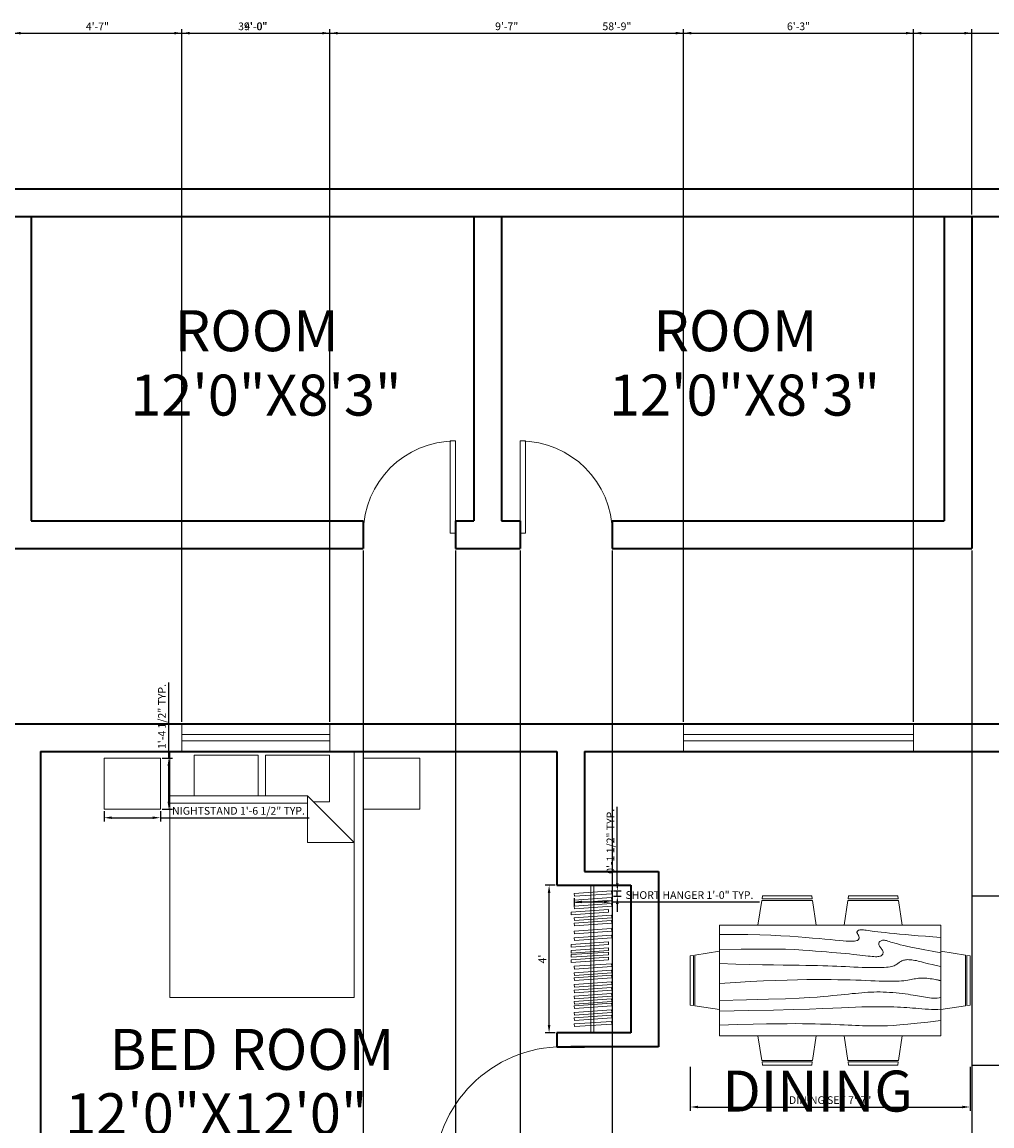
# Model space of a CAD drawing. Units: inches. Extents: x 3412 to 4225, y 13529 to 14581.
# Tile 5 of 7: x 3627 to 3943, y 14222 to 14581. Entities that reach past the tile are written whole.
import ezdxf

# ---------------------------------------------------------------- set-up
doc = ezdxf.new("R2010")
doc.units = ezdxf.units.IN
for name, color, linetype, lineweight in [('A-ANNO-DIMS', 2, 'Continuous', 13), ('A-AREA-IDEN', 7, 'Continuous', 18), ('A-DOOR', 4, 'Continuous', 18), ('A-FLOR-CASE', 9, 'Continuous', 18), ('A-FURN', 8, 'Continuous', 18), ('A-GLAZ', 4, 'Continuous', 13), ('A-WALL', 7, 'Continuous', 35), ('C-SITE-WALL', 7, 'Continuous', 35)]:
    doc.layers.add(name, color=color, linetype=linetype, lineweight=lineweight)
doc.styles.get("Standard").update_dxf_attribs({"font": 'arial.ttf'})
doc.dimstyles.new('ISO-25', dxfattribs={"dimtxt": 2.5, "dimasz": 2.5, "dimexe": 1.25, "dimexo": 0.625, "dimtad": 1, "dimdec": 0, "dimlunit": 3, "dimtxsty": 'Standard', "dimcen": 2.5, "dimadec": 0, "dimazin": 0, "dimtfac": 1, "dimtdec": 0, "dimtmove": 0, "dimatfit": 3, "dimfxl": 1, "dimarcsym": 0})

# ---------------------------------------------------------------- blocks, each defined once
blk = doc.blocks.new('*U3')
for p, q in [((0, 0), (0, -5)), ((30, 0), (30, -5))]:
    blk.add_line(p, q)
blk.add_lwpolyline([(0, 0), (0, 30), (1.75, 30), (1.75, 0)], close=True)
blk.add_arc((0, 0), 30, 0, 90)
blk = doc.blocks.new('Bed - Queen')
for p, q in [((0, -80.00003), (0, 0)), ((0, 0), (59.99999, 0)), ((59.99999, 0), (59.99999, -80.00003)), ((7.99999, -1.2), (28.79998, -1.2)), ((7.99999, -14.4), (7.99999, -1.2)), ((28.79998, -1.2), (28.79998, -14.4)), ((31.19999, -1.2), (51.99999, -1.2)), ((31.19999, -14.4), (31.19999, -1.2)), ((51.99999, -1.2), (51.99999, -16.4)), ((0, -14.4), (44.8, -14.4)), ((44.8, -16.8), (0, -16.8)), ((59.99999, -29.6), (44.8, -14.4)), ((44.8, -14.4), (44.8, -29.6)), ((51.99999, -16.4), (46.79936, -16.4)), ((44.8, -29.6), (59.99999, -29.6)), ((59.99999, -80.00003), (0, -80.00003))]:
    blk.add_line(p, q)
blk = doc.blocks.new('Dining Set - 36 x 72 in.')
for p, q in [((-22.2343, 26.00059), (-23.4847, 17.99762)), ((-22.2304, 26), (-5.7608, 26)), ((-22, 27.5), (-22.1562, 26.50042)), ((-5.8416, 26.5), (-22.1534, 26.5)), ((-22, 27.5), (-6, 27.5)), ((-5.8437, 26.49966), (-6, 27.5)), ((-4.5152, 17.99762), (-5.7655, 25.99926)), ((5.7657, 26.00059), (4.5153, 17.99762)), ((5.7696, 26), (22.2392, 26)), ((6, 27.5), (5.8438, 26.50042)), ((22.1584, 26.5), (5.8466, 26.5)), ((6, 27.5), (22, 27.5)), ((22.1563, 26.49966), (22, 27.5)), ((23.4848, 17.99762), (22.2345, 25.99926)), ((36, 18), (-36, 18)), ((-36, 18), (-36, -18)), ((36, -18), (36, 18)), ((-45.5, 8), (-44.5004, 8.15617)), ((-45.5, 8), (-45.5, -8)), ((-44.5, -8.15843), (-44.5, 8.15338)), ((-44.0006, 8.23428), (-35.9976, 9.48474)), ((-44, 8.23041), (-44, -8.23915)), ((44.0006, 8.23428), (35.9976, 9.48474)), ((44, 8.23041), (44, -8.23915)), ((44.5, -8.15843), (44.5, 8.15338)), ((45.5, 8), (44.5005, 8.15617)), ((45.5, 8), (45.5, -8)), ((-44.4997, -8.15631), (-45.5, -8)), ((-35.9976, -9.48476), (-43.9993, -8.2345)), ((35.9976, -9.48476), (43.9993, -8.2345)), ((44.4997, -8.15631), (45.5, -8)), ((-36, -18), (36, -18)), ((-22.2343, -26.0006), (-23.4847, -17.99762)), ((-4.5152, -17.99762), (-5.7655, -25.99928)), ((5.7657, -26.0006), (4.5153, -17.99762)), ((23.4848, -17.99762), (22.2345, -25.99928)), ((-22.2304, -26), (-5.7608, -26)), ((-22, -27.5), (-22.1562, -26.50044)), ((-5.8416, -26.5), (-22.1534, -26.5)), ((-22, -27.5), (-6, -27.5)), ((-5.8437, -26.49967), (-6, -27.5)), ((5.7696, -26), (22.2392, -26)), ((6, -27.5), (5.8438, -26.50044)), ((22.1584, -26.5), (5.8466, -26.5)), ((6, -27.5), (22, -27.5)), ((22.1563, -26.49967), (22, -27.5))]:
    blk.add_line(p, q)
for points in [[(-36, 15), (-31.1772, 14.97754), (-26.8079, 14.91406), (-22.8538, 14.81543), (-19.276, 14.6875), (-16.0362, 14.53613), (-13.0957, 14.36718), (-10.4159, 14.18652), (-7.9583, 14), (-5.6904, 13.81315), (-3.6035, 13.63021), (-1.6954, 13.45508), (0.0365, 13.29166), (1.5945, 13.14388), (2.9811, 13.01562), (4.1988, 12.9108), (5.25, 12.83333), (6.1393, 12.78613), (6.8802, 12.76823), (7.4883, 12.77767), (7.9792, 12.8125), (8.3685, 12.87077), (8.6719, 12.95052), (8.9049, 13.0498), (9.0833, 13.16666), (9.2205, 13.29899), (9.3216, 13.44401), (9.3895, 13.59879), (9.4271, 13.76041), (9.4373, 13.92594), (9.4232, 14.09245), (9.3875, 14.257), (9.3333, 14.41666), (9.2638, 14.56917), (9.1836, 14.71484), (9.0975, 14.85465), (9.0104, 14.98958), (8.9272, 15.1206), (8.8529, 15.2487), (8.7922, 15.37483), (8.75, 15.5), (8.7305, 15.62467), (8.7344, 15.74739), (8.7617, 15.86621), (8.8125, 15.97916), (8.8867, 16.08431), (8.9844, 16.17968), (9.1055, 16.26334), (9.25, 16.33333), (9.4189, 16.38802), (9.6172, 16.42708), (9.8506, 16.45052), (10.125, 16.45833), (10.4463, 16.45052), (10.8203, 16.42708), (11.2529, 16.38802), (11.75, 16.33333), (12.3184, 16.26318), (12.9694, 16.17838), (13.7151, 16.07991), (14.5677, 15.96875), (15.5395, 15.84586), (16.6426, 15.71224), (17.8893, 15.56884), (19.2917, 15.41666), (20.859, 15.25667), (22.5879, 15.08984), (24.4721, 14.91715), (26.5052, 14.73958), (28.6809, 14.5581), (30.9929, 14.3737), (33.4347, 14.18733), (36, 14)], [(-36, 10), (-28.9766, 10.14274), (-23.1725, 10.20442), (-18.4241, 10.19775), (-14.5677, 10.13541), (-11.4399, 10.03011), (-8.877, 9.89453), (-6.7154, 9.74137), (-4.7917, 9.58333), (-2.9698, 9.43082), (-1.2246, 9.28515), (0.4415, 9.14534), (2.026, 9.01041), (3.5266, 8.87939), (4.9408, 8.7513), (6.266, 8.62516), (7.5, 8.5), (8.6411, 8.37549), (9.6914, 8.2539), (10.6538, 8.13818), (11.5312, 8.03125), (12.3267, 7.93603), (13.043, 7.85547), (13.6831, 7.79248), (14.25, 7.75), (14.7471, 7.7303), (15.1797, 7.73307), (15.5537, 7.75732), (15.875, 7.80208), (16.1494, 7.86637), (16.3828, 7.94922), (16.5811, 8.04964), (16.75, 8.16666), (16.8944, 8.29915), (17.0143, 8.44531), (17.1089, 8.60319), (17.1771, 8.77083), (17.218, 8.94629), (17.2305, 9.1276), (17.2137, 9.31282), (17.1667, 9.5), (17.0895, 9.6875), (16.987, 9.875), (16.8649, 10.0625), (16.7292, 10.25), (16.5856, 10.4375), (16.4401, 10.625), (16.2985, 10.8125), (16.1667, 11), (16.05, 11.18733), (15.9518, 11.3737), (15.8752, 11.5581), (15.8229, 11.73958), (15.798, 11.91715), (15.8034, 12.08984), (15.842, 12.25667), (15.9167, 12.41666), (16.0295, 12.56836), (16.1784, 12.70833), (16.3605, 12.83268), (16.5729, 12.9375), (16.8127, 13.01888), (17.0768, 13.07291), (17.3625, 13.0957), (17.6667, 13.08333), (17.9894, 13.03312), (18.3418, 12.94726), (18.7382, 12.82918), (19.1927, 12.68229), (19.7195, 12.51001), (20.3327, 12.31575), (21.0465, 12.10294), (21.875, 11.875), (22.8357, 11.63354), (23.959, 11.37304), (25.2786, 11.08618), (26.8282, 10.76562), (28.6414, 10.40405), (30.752, 9.99414), (33.1936, 9.52856), (36, 9)], [(-36, 5.5), (-30.7157, 5.3348), (-26.069, 5.20963), (-21.9946, 5.11767), (-18.4271, 5.05208), (-15.3009, 5.00602), (-12.5508, 4.97265), (-10.1112, 4.94515), (-7.9167, 4.91666), (-5.909, 4.88167), (-4.0586, 4.83984), (-2.3429, 4.79215), (-0.7396, 4.73958), (0.7739, 4.6831), (2.22, 4.6237), (3.6213, 4.56233), (5, 4.5), (6.373, 4.43782), (7.7344, 4.3776), (9.0723, 4.32129), (10.375, 4.27083), (11.6309, 4.22819), (12.8281, 4.19531), (13.9551, 4.17415), (15, 4.16666), (15.954, 4.17448), (16.819, 4.19791), (17.6001, 4.23698), (18.3021, 4.29166), (18.9299, 4.36198), (19.4883, 4.44791), (19.9823, 4.54948), (20.4167, 4.66666), (20.7969, 4.79899), (21.1302, 4.94401), (21.4245, 5.09879), (21.6875, 5.26041), (21.9271, 5.42594), (22.1511, 5.59245), (22.3672, 5.757), (22.5834, 5.91666), (22.8065, 6.06868), (23.0404, 6.21093), (23.2879, 6.34147), (23.5521, 6.45833), (23.8358, 6.55957), (24.142, 6.64323), (24.4735, 6.70735), (24.8334, 6.75), (25.2235, 6.76969), (25.642, 6.76692), (26.0858, 6.74267), (26.5521, 6.69791), (27.0379, 6.63362), (27.5404, 6.55078), (28.0565, 6.45036), (28.5834, 6.33333), (29.1242, 6.19987), (29.7071, 6.04687), (30.3661, 5.87044), (31.1354, 5.66666), (32.0493, 5.43164), (33.142, 5.16146), (34.4475, 4.85221), (36, 4.5)], [(-36, -1), (-30.7915, -0.6591), (-26.0195, -0.38216), (-21.6519, -0.16284), (-17.6563, 0.00521), (-14.0005, 0.12833), (-10.6523, 0.21289), (-7.5796, 0.26522), (-4.75, 0.29166), (-2.134, 0.29793), (0.2878, 0.28711), (2.5317, 0.26163), (4.6146, 0.22396), (6.5529, 0.17651), (8.3633, 0.12174), (10.0623, 0.06209), (11.6667, 0), (13.1899, -0.06201), (14.6341, -0.1211), (15.9982, -0.17432), (17.2813, -0.21875), (18.4823, -0.25147), (19.6003, -0.26953), (20.6343, -0.27002), (21.5834, -0.25), (22.4481, -0.20768), (23.2357, -0.14584), (23.9549, -0.06836), (24.6146, 0.02083), (25.2235, 0.11784), (25.7904, 0.21875), (26.3241, 0.31966), (26.8334, 0.41666), (27.3265, 0.50618), (27.8099, 0.58593), (28.2894, 0.65397), (28.7709, 0.70833), (29.2601, 0.74707), (29.763, 0.76823), (30.2855, 0.76985), (30.8334, 0.75), (31.4088, 0.70784), (31.9994, 0.64713), (32.589, 0.57275), (33.1615, 0.48958), (33.7008, 0.4025), (34.1908, 0.3164), (34.6153, 0.23616), (34.9584, 0.16666), (35.2099, 0.11165), (35.3848, 0.07031), (35.504, 0.04069), (35.5886, 0.02083), (35.6594, 0.00879), (35.7377, 0.0026), (35.8442, 0.00032), (36, 0)], [(-36, -6.5), (-27.1843, -6.31267), (-20.084, -6.1263), (-14.469, -5.9419), (-10.1094, -5.76042), (-6.7752, -5.58285), (-4.2363, -5.41016), (-2.2629, -5.24333), (-0.625, -5.08334), (0.8708, -4.93099), (2.2715, -4.78646), (3.5872, -4.64974), (4.8281, -4.52084), (6.0046, -4.39974), (7.127, -4.28646), (8.2053, -4.18099), (9.25, -4.08334), (10.2705, -3.99382), (11.2734, -3.91407), (12.2647, -3.84603), (13.25, -3.79167), (14.2354, -3.75293), (15.2266, -3.73177), (16.2295, -3.73015), (17.25, -3.75), (18.2912, -3.79248), (19.3451, -3.85547), (20.4009, -3.93604), (21.4479, -4.03125), (22.4754, -4.13819), (23.4727, -4.25391), (24.4289, -4.37549), (25.3334, -4.5), (26.1785, -4.62492), (26.9694, -4.74935), (27.7145, -4.87281), (28.4219, -4.99479), (29.1, -5.11483), (29.7572, -5.23242), (30.4016, -5.34709), (31.0417, -5.45834), (31.6837, -5.56437), (32.3262, -5.65821), (32.9658, -5.73153), (33.599, -5.77604), (34.2224, -5.78345), (34.8327, -5.74545), (35.4264, -5.65373), (36, -5.5)], [(-36, -10), (-26.4022, -9.81299), (-18.4675, -9.62891), (-11.9839, -9.45069), (-6.7396, -9.28125), (-2.5226, -9.12354), (0.8789, -8.98047), (3.6769, -8.85498), (6.0833, -8.75), (8.2767, -8.66765), (10.3021, -8.60677), (12.1712, -8.56543), (13.8958, -8.54167), (15.4876, -8.53353), (16.9583, -8.53907), (18.3197, -8.55632), (19.5834, -8.58334), (20.7616, -8.61841), (21.8685, -8.66081), (22.9188, -8.71004), (23.9271, -8.76563), (24.9081, -8.82707), (25.8763, -8.89388), (26.8465, -8.96558), (27.8334, -9.04167), (28.8474, -9.12118), (29.8828, -9.20117), (30.93, -9.27824), (31.9792, -9.34896), (33.0205, -9.40991), (34.0443, -9.45768), (35.0407, -9.48885), (36, -9.5)], [(-36, -14.5), (-30.0881, -14.33513), (-25.0332, -14.21224), (-20.7312, -14.12647), (-17.0781, -14.07292), (-13.97, -14.04671), (-11.3027, -14.04297), (-8.9724, -14.05681), (-6.875, -14.08334), (-4.9224, -14.11833), (-3.0905, -14.16016), (-1.3709, -14.20785), (0.2448, -14.26042), (1.7647, -14.3169), (3.1973, -14.3763), (4.5507, -14.43767), (5.8333, -14.5), (7.0554, -14.5621), (8.235, -14.62175), (9.3922, -14.67652), (10.5469, -14.72396), (11.7192, -14.76164), (12.929, -14.78711), (14.1965, -14.79794), (15.5417, -14.79167), (16.9933, -14.76424), (18.6152, -14.70508), (20.4804, -14.60197), (22.6615, -14.44271), (25.2312, -14.21509), (28.2624, -13.9069), (31.8277, -13.50594), (36, -13)]]:
    blk.add_lwpolyline(points)
blk = doc.blocks.new('*D15')
at = {"layer": 'A-ANNO-DIMS', "color": 0, "lineweight": -2, "transparency": 16777216}
for p, q in [((3800.73, 14299.93), (3797.55, 14299.93)), ((3798.8, 14254.43), (3798.8, 14297.43)), ((3800.73, 14251.93), (3797.55, 14251.93))]:
    blk.add_line(p, q, dxfattribs=at)
at = {"layer": 'A-ANNO-DIMS', "color": 0, "transparency": 16777216}
for points in [[(3798.38, 14297.43), (3799.21, 14297.43), (3798.8, 14299.93)], [(3798.38, 14254.43), (3799.21, 14254.43), (3798.8, 14251.93)]]:
    blk.add_solid(points, dxfattribs=at)
at = {"layer": 'Defpoints', "color": 0, "transparency": 16777216}
for p in [(3798.8, 14299.93), (3801.36, 14299.93), (3801.36, 14251.93)]:
    blk.add_point(p, dxfattribs=at)
at = {"layer": 'A-ANNO-DIMS', "color": 0, "transparency": 16777216, "insert": (3796.92, 14275.93), "char_height": 2.5, "attachment_point": 5, "rotation": 90}
blk.add_mtext("4'", dxfattribs=at)
blk = doc.blocks.new('NIGHTSTAND')
blk.add_lwpolyline([(0, 16.62), (18.31, 16.62), (18.31, 0), (0, 0)], close=True)
blk = doc.blocks.new('CLOSET-HANGER-SHORT')
blk.add_lwpolyline([(0, 0.87), (12.13, 1.73), (12.19, 0.86), (0.06, 0)], close=True)
blk = doc.blocks.new('*D36')
at = {"layer": 'A-ANNO-DIMS', "color": 0, "lineweight": -2, "transparency": 16777216}
for p, q in [((3654.03, 14324.02), (3654.03, 14320.64)), ((3672.34, 14324.02), (3672.34, 14320.64)), ((3656.53, 14321.89), (3669.84, 14321.89)), ((3672.34, 14321.89), (3720.71, 14321.89))]:
    blk.add_line(p, q, dxfattribs=at)
at = {"layer": 'A-ANNO-DIMS', "color": 0, "transparency": 16777216}
for points in [[(3656.53, 14322.31), (3656.53, 14321.48), (3654.03, 14321.89)], [(3669.84, 14322.31), (3669.84, 14321.48), (3672.34, 14321.89)]]:
    blk.add_solid(points, dxfattribs=at)
at = {"layer": 'Defpoints', "color": 0, "transparency": 16777216}
for p in [(3654.03, 14324.64), (3672.34, 14324.64), (3672.34, 14321.89)]:
    blk.add_point(p, dxfattribs=at)
at = {"layer": 'A-ANNO-DIMS', "color": 0, "transparency": 16777216, "insert": (3697.77, 14323.81), "char_height": 2.5, "attachment_point": 5}
blk.add_mtext('NIGHTSTAND 1\'-6 1/2" TYP.', dxfattribs=at)
blk = doc.blocks.new('*D37')
at = {"layer": 'A-ANNO-DIMS', "color": 0, "lineweight": -2, "transparency": 16777216}
for p, q in [((3675.09, 14341.26), (3675.09, 14365.84)), ((3672.97, 14341.26), (3676.34, 14341.26)), ((3675.09, 14327.14), (3675.09, 14338.76)), ((3672.97, 14324.64), (3676.34, 14324.64))]:
    blk.add_line(p, q, dxfattribs=at)
at = {"layer": 'A-ANNO-DIMS', "color": 0, "transparency": 16777216}
for points in [[(3674.67, 14338.76), (3675.5, 14338.76), (3675.09, 14341.26)], [(3674.67, 14327.14), (3675.5, 14327.14), (3675.09, 14324.64)]]:
    blk.add_solid(points, dxfattribs=at)
at = {"layer": 'Defpoints', "color": 0, "transparency": 16777216}
for p in [(3672.34, 14341.26), (3675.09, 14341.26), (3672.34, 14324.64)]:
    blk.add_point(p, dxfattribs=at)
at = {"layer": 'A-ANNO-DIMS', "color": 0, "transparency": 16777216, "insert": (3673.17, 14354.8), "char_height": 2.5, "attachment_point": 5, "rotation": 90}
blk.add_mtext('1\'-4 1/2" TYP.', dxfattribs=at)
blk = doc.blocks.new('*D42')
at = {"layer": 'A-ANNO-DIMS', "color": 0, "lineweight": -2, "transparency": 16777216}
for p, q in [((3806.97, 14295.71), (3806.97, 14293.26)), ((3809.47, 14294.51), (3816.66, 14294.51)), ((3819.16, 14295.71), (3819.16, 14293.26)), ((3819.16, 14294.51), (3867.25, 14294.51))]:
    blk.add_line(p, q, dxfattribs=at)
at = {"layer": 'A-ANNO-DIMS', "color": 0, "transparency": 16777216}
for points in [[(3809.47, 14294.92), (3809.47, 14294.09), (3806.97, 14294.51)], [(3816.66, 14294.92), (3816.66, 14294.09), (3819.16, 14294.51)]]:
    blk.add_solid(points, dxfattribs=at)
at = {"layer": 'Defpoints', "color": 0, "transparency": 16777216}
for p in [(3806.97, 14296.33), (3819.16, 14296.33), (3819.16, 14294.51)]:
    blk.add_point(p, dxfattribs=at)
at = {"layer": 'A-ANNO-DIMS', "color": 0, "transparency": 16777216, "insert": (3844.45, 14296.42), "char_height": 2.5, "attachment_point": 5}
blk.add_mtext('SHORT HANGER 1\'-0" TYP.', dxfattribs=at)
blk = doc.blocks.new('*D43')
at = {"layer": 'A-ANNO-DIMS', "color": 0, "lineweight": -2, "transparency": 16777216}
for p, q in [((3820.99, 14300.57), (3820.99, 14325.38)), ((3819.79, 14298.07), (3822.24, 14298.07)), ((3819.79, 14296.33), (3822.24, 14296.33)), ((3820.99, 14296.33), (3820.99, 14298.07)), ((3820.99, 14293.83), (3820.99, 14291.33))]:
    blk.add_line(p, q, dxfattribs=at)
at = {"layer": 'A-ANNO-DIMS', "color": 0, "transparency": 16777216}
for points in [[(3820.57, 14300.57), (3821.41, 14300.57), (3820.99, 14298.07)], [(3820.57, 14293.83), (3821.41, 14293.83), (3820.99, 14296.33)]]:
    blk.add_solid(points, dxfattribs=at)
at = {"layer": 'Defpoints', "color": 0, "transparency": 16777216}
for p in [(3819.16, 14298.07), (3819.16, 14296.33), (3820.99, 14298.07)]:
    blk.add_point(p, dxfattribs=at)
at = {"layer": 'A-ANNO-DIMS', "color": 0, "transparency": 16777216, "insert": (3819.07, 14314.22), "char_height": 2.5, "attachment_point": 5, "rotation": 90}
blk.add_mtext('0\'-1 1/2" TYP.', dxfattribs=at)
blk = doc.blocks.new('*D52')
at = {"layer": 'A-ANNO-DIMS', "color": 0, "lineweight": -2, "transparency": 16777216}
for p, q in [((3844.72, 14240.84), (3844.72, 14226.56)), ((3935.72, 14240.84), (3935.72, 14226.56)), ((3847.22, 14227.81), (3933.22, 14227.81))]:
    blk.add_line(p, q, dxfattribs=at)
at = {"layer": 'A-ANNO-DIMS', "color": 0, "transparency": 16777216}
for points in [[(3847.22, 14228.23), (3847.22, 14227.4), (3844.72, 14227.81)], [(3933.22, 14228.23), (3933.22, 14227.4), (3935.72, 14227.81)]]:
    blk.add_solid(points, dxfattribs=at)
at = {"layer": 'Defpoints', "color": 0, "transparency": 16777216}
for p in [(3844.72, 14241.46), (3935.72, 14241.46), (3935.72, 14227.81)]:
    blk.add_point(p, dxfattribs=at)
at = {"layer": 'A-ANNO-DIMS', "color": 0, "transparency": 16777216, "insert": (3890.22, 14229.73), "char_height": 2.5, "attachment_point": 5}
blk.add_mtext('DINING SET 7\'-7"', dxfattribs=at)
blk = doc.blocks.new('*D53')
at = {"layer": 'A-ANNO-DIMS', "color": 0, "lineweight": -2, "transparency": 16777216}
for p, q in [((3936.34, 14296.46), (3950.62, 14296.46)), ((3949.37, 14243.96), (3949.37, 14293.96)), ((3936.34, 14241.46), (3950.62, 14241.46))]:
    blk.add_line(p, q, dxfattribs=at)
at = {"layer": 'A-ANNO-DIMS', "color": 0, "transparency": 16777216}
for points in [[(3948.95, 14293.96), (3949.79, 14293.96), (3949.37, 14296.46)], [(3948.95, 14243.96), (3949.79, 14243.96), (3949.37, 14241.46)]]:
    blk.add_solid(points, dxfattribs=at)
at = {"layer": 'Defpoints', "color": 0, "transparency": 16777216}
for p in [(3935.72, 14296.46), (3949.37, 14296.46), (3935.72, 14241.46)]:
    blk.add_point(p, dxfattribs=at)
at = {"layer": 'A-ANNO-DIMS', "color": 0, "transparency": 16777216, "insert": (3947.49, 14268.96), "char_height": 2.5, "attachment_point": 5, "rotation": 90}
blk.add_mtext('4\'-7"', dxfattribs=at)
blk = doc.blocks.new('*D56')
at = {"layer": 'A-ANNO-DIMS', "color": 0, "lineweight": -2, "transparency": 16777216}
for p, q in [((3468.36, 14527.06), (3468.36, 14578.28)), ((4173.36, 14527.06), (4173.36, 14578.28)), ((3470.86, 14577.03), (4170.86, 14577.03))]:
    blk.add_line(p, q, dxfattribs=at)
at = {"layer": 'A-ANNO-DIMS', "color": 0, "transparency": 16777216}
for points in [[(3470.86, 14577.45), (3470.86, 14576.62), (3468.36, 14577.03)], [(4170.86, 14577.45), (4170.86, 14576.62), (4173.36, 14577.03)]]:
    blk.add_solid(points, dxfattribs=at)
at = {"layer": 'Defpoints', "color": 0, "transparency": 16777216}
for p in [(4173.36, 14577.03), (3468.36, 14526.43), (4173.36, 14526.43)]:
    blk.add_point(p, dxfattribs=at)
at = {"layer": 'A-ANNO-DIMS', "color": 0, "transparency": 16777216, "insert": (3820.86, 14578.93), "char_height": 2.5, "attachment_point": 5}
blk.add_mtext('58\'-9"', dxfattribs=at)
blk = doc.blocks.new('*D59')
at = {"layer": 'A-ANNO-DIMS', "color": 0, "lineweight": -2, "transparency": 16777216}
for p, q in [((3468.36, 14527.06), (3468.36, 14578.28)), ((3936.36, 14518.06), (3936.36, 14578.28)), ((3470.86, 14577.03), (3933.86, 14577.03))]:
    blk.add_line(p, q, dxfattribs=at)
at = {"layer": 'A-ANNO-DIMS', "color": 0, "transparency": 16777216}
for points in [[(3470.86, 14577.45), (3470.86, 14576.62), (3468.36, 14577.03)], [(3933.86, 14577.45), (3933.86, 14576.62), (3936.36, 14577.03)]]:
    blk.add_solid(points, dxfattribs=at)
at = {"layer": 'Defpoints', "color": 0, "transparency": 16777216}
for p in [(3936.36, 14577.03), (3468.36, 14526.43), (3936.36, 14517.43)]:
    blk.add_point(p, dxfattribs=at)
at = {"layer": 'A-ANNO-DIMS', "color": 0, "transparency": 16777216, "insert": (3702.36, 14578.93), "char_height": 2.5, "attachment_point": 5}
blk.add_mtext('39\'-0"', dxfattribs=at)
blk = doc.blocks.new('*D63')
at = {"layer": 'A-ANNO-DIMS', "color": 0, "lineweight": -2, "transparency": 16777216}
for p, q in [((3615.36, 14408.81), (3615.36, 13550.58)), ((3738.36, 14408.81), (3738.36, 13550.58)), ((3617.86, 13551.83), (3735.86, 13551.83))]:
    blk.add_line(p, q, dxfattribs=at)
at = {"layer": 'A-ANNO-DIMS', "color": 0, "transparency": 16777216}
for points in [[(3617.86, 13552.25), (3617.86, 13551.42), (3615.36, 13551.83)], [(3735.86, 13552.25), (3735.86, 13551.42), (3738.36, 13551.83)]]:
    blk.add_solid(points, dxfattribs=at)
at = {"layer": 'Defpoints', "color": 0, "transparency": 16777216}
for p in [(3615.36, 14409.43), (3738.36, 14409.43), (3738.36, 13551.83)]:
    blk.add_point(p, dxfattribs=at)
at = {"layer": 'A-ANNO-DIMS', "color": 0, "transparency": 16777216, "insert": (3676.86, 13553.73), "char_height": 2.5, "attachment_point": 5}
blk.add_mtext('10\'-3"', dxfattribs=at)
blk = doc.blocks.new('*D64')
at = {"layer": 'A-ANNO-DIMS', "color": 0, "lineweight": -2, "transparency": 16777216}
for p, q in [((3738.36, 14408.81), (3738.36, 13550.58)), ((3768.36, 14408.81), (3768.36, 13550.58)), ((3740.86, 13551.83), (3765.86, 13551.83))]:
    blk.add_line(p, q, dxfattribs=at)
at = {"layer": 'A-ANNO-DIMS', "color": 0, "transparency": 16777216}
for points in [[(3740.86, 13552.25), (3740.86, 13551.42), (3738.36, 13551.83)], [(3765.86, 13552.25), (3765.86, 13551.42), (3768.36, 13551.83)]]:
    blk.add_solid(points, dxfattribs=at)
at = {"layer": 'Defpoints', "color": 0, "transparency": 16777216}
for p in [(3738.36, 14409.43), (3768.36, 14409.43), (3768.36, 13551.83)]:
    blk.add_point(p, dxfattribs=at)
at = {"layer": 'A-ANNO-DIMS', "color": 0, "transparency": 16777216, "insert": (3753.36, 13553.73), "char_height": 2.5, "attachment_point": 5}
blk.add_mtext('2\'-6"', dxfattribs=at)
blk = doc.blocks.new('*D65')
at = {"layer": 'A-ANNO-DIMS', "color": 0, "lineweight": -2, "transparency": 16777216}
for p, q in [((3768.36, 14408.81), (3768.36, 13550.58)), ((3789.36, 14408.81), (3789.36, 13550.58)), ((3770.86, 13551.83), (3786.86, 13551.83))]:
    blk.add_line(p, q, dxfattribs=at)
at = {"layer": 'A-ANNO-DIMS', "color": 0, "transparency": 16777216}
for points in [[(3770.86, 13552.25), (3770.86, 13551.42), (3768.36, 13551.83)], [(3786.86, 13552.25), (3786.86, 13551.42), (3789.36, 13551.83)]]:
    blk.add_solid(points, dxfattribs=at)
at = {"layer": 'Defpoints', "color": 0, "transparency": 16777216}
for p in [(3768.36, 14409.43), (3789.36, 14409.43), (3789.36, 13551.83)]:
    blk.add_point(p, dxfattribs=at)
at = {"layer": 'A-ANNO-DIMS', "color": 0, "transparency": 16777216, "insert": (3778.86, 13553.73), "char_height": 2.5, "attachment_point": 5}
blk.add_mtext('1\'-9"', dxfattribs=at)
blk = doc.blocks.new('*D66')
at = {"layer": 'A-ANNO-DIMS', "color": 0, "lineweight": -2, "transparency": 16777216}
for p, q in [((3789.36, 14408.81), (3789.36, 13550.58)), ((3819.36, 14408.81), (3819.36, 13550.58)), ((3791.86, 13551.83), (3816.86, 13551.83))]:
    blk.add_line(p, q, dxfattribs=at)
at = {"layer": 'A-ANNO-DIMS', "color": 0, "transparency": 16777216}
for points in [[(3791.86, 13552.25), (3791.86, 13551.42), (3789.36, 13551.83)], [(3816.86, 13552.25), (3816.86, 13551.42), (3819.36, 13551.83)]]:
    blk.add_solid(points, dxfattribs=at)
at = {"layer": 'Defpoints', "color": 0, "transparency": 16777216}
for p in [(3789.36, 14409.43), (3819.36, 14409.43), (3819.36, 13551.83)]:
    blk.add_point(p, dxfattribs=at)
at = {"layer": 'A-ANNO-DIMS', "color": 0, "transparency": 16777216, "insert": (3804.36, 13553.73), "char_height": 2.5, "attachment_point": 5}
blk.add_mtext('2\'-6"', dxfattribs=at)
blk = doc.blocks.new('*D67')
at = {"layer": 'A-ANNO-DIMS', "color": 0, "lineweight": -2, "transparency": 16777216}
for p, q in [((3819.36, 14408.81), (3819.36, 13550.58)), ((3936.36, 14408.81), (3936.36, 13550.58)), ((3821.86, 13551.83), (3933.86, 13551.83))]:
    blk.add_line(p, q, dxfattribs=at)
at = {"layer": 'A-ANNO-DIMS', "color": 0, "transparency": 16777216}
for points in [[(3821.86, 13552.25), (3821.86, 13551.42), (3819.36, 13551.83)], [(3933.86, 13552.25), (3933.86, 13551.42), (3936.36, 13551.83)]]:
    blk.add_solid(points, dxfattribs=at)
at = {"layer": 'Defpoints', "color": 0, "transparency": 16777216}
for p in [(3819.36, 14409.43), (3936.36, 14409.43), (3936.36, 13551.83)]:
    blk.add_point(p, dxfattribs=at)
at = {"layer": 'A-ANNO-DIMS', "color": 0, "transparency": 16777216, "insert": (3877.86, 13553.73), "char_height": 2.5, "attachment_point": 5}
blk.add_mtext('9\'-9"', dxfattribs=at)
blk = doc.blocks.new('*D68')
at = {"layer": 'A-ANNO-DIMS', "color": 0, "lineweight": -2, "transparency": 16777216}
for p, q in [((3624.36, 14353.06), (3624.36, 14578.28)), ((3679.38, 14353.06), (3679.38, 14578.28)), ((3626.86, 14577.03), (3676.88, 14577.03))]:
    blk.add_line(p, q, dxfattribs=at)
at = {"layer": 'A-ANNO-DIMS', "color": 0, "transparency": 16777216}
for points in [[(3626.86, 14577.45), (3626.86, 14576.62), (3624.36, 14577.03)], [(3676.88, 14577.45), (3676.88, 14576.62), (3679.38, 14577.03)]]:
    blk.add_solid(points, dxfattribs=at)
at = {"layer": 'Defpoints', "color": 0, "transparency": 16777216}
for p in [(3679.38, 14577.03), (3624.36, 14352.43), (3679.38, 14352.43)]:
    blk.add_point(p, dxfattribs=at)
at = {"layer": 'A-ANNO-DIMS', "color": 0, "transparency": 16777216, "insert": (3651.87, 14578.91), "char_height": 2.5, "attachment_point": 5}
blk.add_mtext('4\'-7"', dxfattribs=at)
blk = doc.blocks.new('*D69')
at = {"layer": 'A-ANNO-DIMS', "color": 0, "lineweight": -2, "transparency": 16777216}
for p, q in [((3679.38, 14353.06), (3679.38, 14578.28)), ((3727.48, 14353.06), (3727.48, 14578.28)), ((3681.88, 14577.03), (3724.98, 14577.03))]:
    blk.add_line(p, q, dxfattribs=at)
at = {"layer": 'A-ANNO-DIMS', "color": 0, "transparency": 16777216}
for points in [[(3681.88, 14577.45), (3681.88, 14576.62), (3679.38, 14577.03)], [(3724.98, 14577.45), (3724.98, 14576.62), (3727.48, 14577.03)]]:
    blk.add_solid(points, dxfattribs=at)
at = {"layer": 'Defpoints', "color": 0, "transparency": 16777216}
for p in [(3727.48, 14577.03), (3679.38, 14352.43), (3727.48, 14352.43)]:
    blk.add_point(p, dxfattribs=at)
at = {"layer": 'A-ANNO-DIMS', "color": 0, "transparency": 16777216, "insert": (3703.43, 14578.93), "char_height": 2.5, "attachment_point": 5}
blk.add_mtext('4\'-0"', dxfattribs=at)
blk = doc.blocks.new('*D70')
at = {"layer": 'A-ANNO-DIMS', "color": 0, "lineweight": -2, "transparency": 16777216}
for p, q in [((3727.48, 14353.06), (3727.48, 14578.28)), ((3842.52, 14353.06), (3842.52, 14578.28)), ((3729.98, 14577.03), (3840.02, 14577.03))]:
    blk.add_line(p, q, dxfattribs=at)
at = {"layer": 'A-ANNO-DIMS', "color": 0, "transparency": 16777216}
for points in [[(3729.98, 14577.45), (3729.98, 14576.62), (3727.48, 14577.03)], [(3840.02, 14577.45), (3840.02, 14576.62), (3842.52, 14577.03)]]:
    blk.add_solid(points, dxfattribs=at)
at = {"layer": 'Defpoints', "color": 0, "transparency": 16777216}
for p in [(3842.52, 14577.03), (3727.48, 14352.43), (3842.52, 14352.43)]:
    blk.add_point(p, dxfattribs=at)
at = {"layer": 'A-ANNO-DIMS', "color": 0, "transparency": 16777216, "insert": (3785, 14578.93), "char_height": 2.5, "attachment_point": 5}
blk.add_mtext('9\'-7"', dxfattribs=at)
blk = doc.blocks.new('*D71')
at = {"layer": 'A-ANNO-DIMS', "color": 0, "lineweight": -2, "transparency": 16777216}
for p, q in [((3842.52, 14353.06), (3842.52, 14578.28)), ((3917.36, 14353.06), (3917.36, 14578.28)), ((3845.02, 14577.03), (3914.86, 14577.03))]:
    blk.add_line(p, q, dxfattribs=at)
at = {"layer": 'A-ANNO-DIMS', "color": 0, "transparency": 16777216}
for points in [[(3845.02, 14577.45), (3845.02, 14576.62), (3842.52, 14577.03)], [(3914.86, 14577.45), (3914.86, 14576.62), (3917.36, 14577.03)]]:
    blk.add_solid(points, dxfattribs=at)
at = {"layer": 'Defpoints', "color": 0, "transparency": 16777216}
for p in [(3917.36, 14577.03), (3842.52, 14352.43), (3917.36, 14352.43)]:
    blk.add_point(p, dxfattribs=at)
at = {"layer": 'A-ANNO-DIMS', "color": 0, "transparency": 16777216, "insert": (3879.94, 14578.93), "char_height": 2.5, "attachment_point": 5}
blk.add_mtext('6\'-3"', dxfattribs=at)
blk = doc.blocks.new('*D72')
at = {"layer": 'A-ANNO-DIMS', "color": 0, "lineweight": -2, "transparency": 16777216}
for p, q in [((3917.36, 14353.06), (3917.36, 14578.28)), ((4092.36, 14353.06), (4092.36, 14578.28)), ((3919.86, 14577.03), (4089.86, 14577.03))]:
    blk.add_line(p, q, dxfattribs=at)
at = {"layer": 'A-ANNO-DIMS', "color": 0, "transparency": 16777216}
for points in [[(3919.86, 14577.45), (3919.86, 14576.62), (3917.36, 14577.03)], [(4089.86, 14577.45), (4089.86, 14576.62), (4092.36, 14577.03)]]:
    blk.add_solid(points, dxfattribs=at)
at = {"layer": 'Defpoints', "color": 0, "transparency": 16777216}
for p in [(4092.36, 14577.03), (3917.36, 14352.43), (4092.36, 14352.43)]:
    blk.add_point(p, dxfattribs=at)
at = {"layer": 'A-ANNO-DIMS', "color": 0, "transparency": 16777216, "insert": (4004.86, 14578.91), "char_height": 2.5, "attachment_point": 5}
blk.add_mtext('14\'-7"', dxfattribs=at)

msp = doc.modelspace()

# ---------------------------------------------------------------- linework, layer by layer
at = {"layer": 'A-FLOR-CASE'}
for p, q in [((3812.36, 14299.93), (3812.36, 14251.93)), ((3813.36, 14299.93), (3813.36, 14251.93))]:
    msp.add_line(p, q, dxfattribs=at)
at = {"layer": 'A-GLAZ'}
for p, q in [((3679.38, 14343.43), (3679.38, 14352.43)), ((3727.48, 14343.43), (3727.48, 14352.43)), ((3842.52, 14343.43), (3842.52, 14352.43)), ((3917.36, 14343.43), (3917.36, 14352.43)), ((3679.38, 14348.93), (3727.48, 14348.93)), ((3842.52, 14348.93), (3917.36, 14348.93)), ((3679.38, 14346.93), (3727.48, 14346.93)), ((3842.52, 14346.93), (3917.36, 14346.93))]:
    msp.add_line(p, q, dxfattribs=at)
at = {"layer": 'A-WALL'}
for p, q in [((3630.36, 14517.43), (3630.36, 14418.43)), ((3774.36, 14517.43), (3774.36, 14418.43)), ((3783.36, 14517.43), (3783.36, 14418.43)), ((3927.36, 14517.43), (3927.36, 14418.43)), ((3936.36, 14517.43), (3936.36, 14409.43)), ((3630.36, 14418.43), (3738.36, 14418.43)), ((3738.36, 14418.43), (3738.36, 14409.43)), ((3768.36, 14418.43), (3768.36, 14409.43)), ((3768.36, 14418.43), (3774.36, 14418.43)), ((3783.36, 14418.43), (3789.36, 14418.43)), ((3789.36, 14418.43), (3789.36, 14409.43)), ((3819.36, 14418.43), (3819.36, 14409.43)), ((3819.36, 14418.43), (3927.36, 14418.43)), ((3615.36, 14409.43), (3738.36, 14409.43)), ((3768.36, 14409.43), (3789.36, 14409.43)), ((3819.36, 14409.43), (3936.36, 14409.43)), ((3624.36, 14352.43), (4092.36, 14352.43)), ((3633.36, 14343.43), (3633.36, 14199.43)), ((3633.36, 14343.43), (3801.36, 14343.43)), ((3801.36, 14343.43), (3801.36, 14299.93)), ((3810.36, 14343.43), (3810.36, 14304.43)), ((3810.36, 14343.43), (3948.36, 14343.43)), ((3810.36, 14304.43), (3834.36, 14304.43)), ((3834.36, 14304.43), (3834.36, 14247.43)), ((3801.36, 14299.93), (3825.36, 14299.93)), ((3825.36, 14299.93), (3825.36, 14251.93)), ((3825.36, 14251.93), (3801.36, 14251.93)), ((3801.36, 14251.93), (3801.36, 14247.43)), ((3801.36, 14247.43), (3810.36, 14247.43)), ((3834.36, 14247.43), (3805.86, 14247.43))]:
    msp.add_line(p, q, dxfattribs=at)
at = {"layer": 'C-SITE-WALL'}
for p, q in [((3468.36, 14526.43), (4173.36, 14526.43)), ((3477.36, 14517.43), (4164.36, 14517.43))]:
    msp.add_line(p, q, dxfattribs=at)

# ---------------------------------------------------------------- block references
at = {"layer": 'A-DOOR', "xscale": -1}
msp.add_blockref('*U3', (3768.36, 14414.43), dxfattribs=at)
at = {"layer": 'A-DOOR'}
msp.add_blockref('*U3', (3789.36, 14414.43), dxfattribs=at)
at = {"layer": 'A-DOOR', "xscale": 1.399999999999999, "yscale": 1.399999999999999, "zscale": 1.399999999999999, "rotation": 89.99999999999999}
msp.add_blockref('*U3', (3803.36, 14205.43), dxfattribs=at)
at = {"layer": 'A-FLOR-CASE'}
for p in [(3806.97, 14296.33), (3806.97, 14294.21), (3805.97, 14290.33), (3806.97, 14292.29), (3806.97, 14288.49), (3806.97, 14286.72), (3806.97, 14284.17), (3805.97, 14279.75), (3806.97, 14281.93), (3805.97, 14277.89), (3805.97, 14276.49), (3805.97, 14274.8), (3806.97, 14272.69), (3806.97, 14270.63), (3806.97, 14268.94), (3806.97, 14266.79), (3806.97, 14264.97), (3806.97, 14263.04), (3806.97, 14261.25), (3806.97, 14259.83), (3806.97, 14257.73), (3806.97, 14255.99), (3806.97, 14253.94)]:
    msp.add_blockref('CLOSET-HANGER-SHORT', p, dxfattribs=at)
at = {"layer": 'A-FURN'}
for name, p in [('NIGHTSTAND', (3654.03, 14324.64)), ('Bed - Queen', (3675.39, 14343.43)), ('Dining Set - 36 x 72 in.', (3890.22, 14268.96))]:
    msp.add_blockref(name, p, dxfattribs=at)
at = {"layer": 'A-FURN', "extrusion": (0, 0, -1), "zscale": -1}
msp.add_blockref('NIGHTSTAND', (-3756.75, 14324.64), dxfattribs=at)

# ---------------------------------------------------------------- texts
at = {"layer": 'A-AREA-IDEN'}
for s, height, p in [('ROOM', 13.329, (3677.05, 14473.59)), ('ROOM', 13.329, (3832.76, 14473.59)), ('12\'0"X8\'3"', 13.329, (3662.56, 14452.66)), ('12\'0"X8\'3"', 13.329, (3818.26, 14452.66)), ('BED ROOM', 13.329, (3655.86, 14239.89)), ('DINING', 13.329, (3855.17, 14226.32)), ('12\'0"X12\'0"', 13.3293, (3641.36, 14218.95))]:
    msp.add_text(s, height=height, dxfattribs=at).set_placement(p)

# ---------------------------------------------------------------- dimensions: what is measured, and where the dimension line sits
at = {"layer": 'A-ANNO-DIMS'}
for base, p1, p2, picture, middle in [((4173.36, 14577.03), (3468.36, 14526.43), (4173.36, 14526.43), '*D56', (3820.86, 14578.93)), ((3936.36, 14577.03), (3468.36, 14526.43), (3936.36, 14517.43), '*D59', (3702.36, 14578.93)), ((3679.38, 14577.03), (3624.36, 14352.43), (3679.38, 14352.43), '*D68', (3651.87, 14578.91)), ((3727.48, 14577.03), (3679.38, 14352.43), (3727.48, 14352.43), '*D69', (3703.43, 14578.93)), ((3842.52, 14577.03), (3727.48, 14352.43), (3842.52, 14352.43), '*D70', (3785, 14578.93)), ((3917.36, 14577.03), (3842.52, 14352.43), (3917.36, 14352.43), '*D71', (3879.94, 14578.93)), ((4092.36, 14577.03), (3917.36, 14352.43), (4092.36, 14352.43), '*D72', (4004.86, 14578.91)), ((3738.36, 13551.83), (3615.36, 14409.43), (3738.36, 14409.43), '*D63', (3676.86, 13553.73)), ((3768.36, 13551.83), (3738.36, 14409.43), (3768.36, 14409.43), '*D64', (3753.36, 13553.73)), ((3789.36, 13551.83), (3768.36, 14409.43), (3789.36, 14409.43), '*D65', (3778.86, 13553.73)), ((3819.36, 13551.83), (3789.36, 14409.43), (3819.36, 14409.43), '*D66', (3804.36, 13553.73)), ((3936.36, 13551.83), (3819.36, 14409.43), (3936.36, 14409.43), '*D67', (3877.86, 13553.73))]:
    dim = msp.add_linear_dim(base=base, p1=p1, p2=p2, dimstyle='ISO-25', override={"dimdec": 1, "dimlfac": 1, "dimrnd": 0, "dimzin": 1, "dimdsep": 46, "dimlunit": 4, "dimfrac": 2}, dxfattribs=at)
    dim.commit()
    dim.dimension.update_dxf_attribs({"geometry": picture, "text_midpoint": middle})
for base, p1, p2, picture, middle in [((3675.09, 14341.26), (3672.34, 14324.64), (3672.34, 14341.26), '*D37', (3673.17, 14354.8)), ((3820.99, 14298.07), (3819.16, 14296.33), (3819.16, 14298.07), '*D43', (3819.07, 14314.22))]:
    dim = msp.add_linear_dim(base=base, p1=p1, p2=p2, angle=90, text='<> TYP.', dimstyle='ISO-25', override={"dimdec": 1, "dimlfac": 1, "dimrnd": 0, "dimzin": 1, "dimdsep": 46, "dimlunit": 4, "dimfrac": 2}, dxfattribs=at)
    dim.commit()
    dim.dimension.update_dxf_attribs({"geometry": picture, "text_midpoint": middle})
for base, p1, p2, text, picture, middle in [((3672.34, 14321.89), (3654.03, 14324.64), (3672.34, 14324.64), 'NIGHTSTAND <> TYP.', '*D36', (3697.77, 14323.81)), ((3819.16, 14294.51), (3806.97, 14296.33), (3819.16, 14296.33), 'SHORT HANGER <> TYP.', '*D42', (3844.45, 14296.42)), ((3935.72, 14227.81), (3844.72, 14241.46), (3935.72, 14241.46), 'DINING SET <>', '*D52', (3890.22, 14229.73))]:
    dim = msp.add_linear_dim(base=base, p1=p1, p2=p2, text=text, dimstyle='ISO-25', override={"dimdec": 1, "dimlfac": 1, "dimrnd": 0, "dimzin": 1, "dimdsep": 46, "dimlunit": 4, "dimfrac": 2}, dxfattribs=at)
    dim.commit()
    dim.dimension.update_dxf_attribs({"geometry": picture, "text_midpoint": middle})
for base, p1, p2, override, picture, middle in [((3798.8, 14299.93), (3801.36, 14251.93), (3801.36, 14299.93), {"dimclrd": 0, "dimclre": 0, "dimclrt": 0}, '*D15', (3796.92, 14275.93)), ((3949.37, 14296.46), (3935.72, 14241.46), (3935.72, 14296.46), {"dimdec": 1, "dimlfac": 1, "dimrnd": 0, "dimzin": 1, "dimdsep": 46, "dimlunit": 4, "dimfrac": 2}, '*D53', (3947.49, 14268.96))]:
    dim = msp.add_linear_dim(base=base, p1=p1, p2=p2, angle=90, dimstyle='ISO-25', override=override, dxfattribs=at)
    dim.commit()
    dim.dimension.update_dxf_attribs({"geometry": picture, "text_midpoint": middle})

doc.saveas('drawing.dxf')
